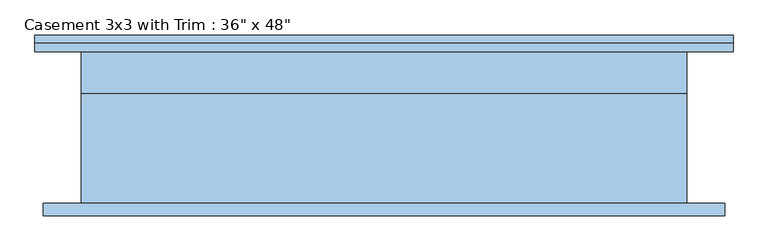
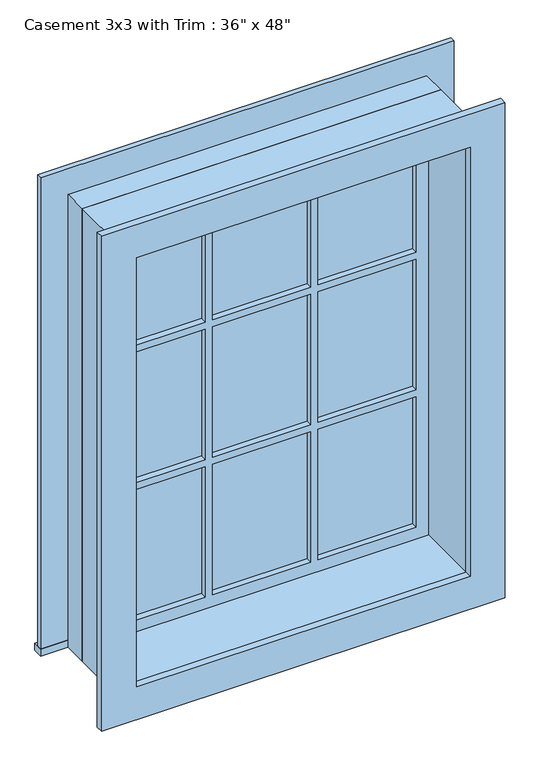
"""IFC4 building model written with IfcOpenShell, lengths in millimetres: window geometry."""

from ifc_helpers import new_model, si_unit, frame, origin, place, context, project, spatial, polyline, outline, extrude, source, transform, mapped, element, save


def window_b7d400b3(model_context):
    return source(origin(), model_context, "Body", "SweptSolid", [
        extrude(outline(polyline([(-527.05, 139.7), (527.05, 139.7), (527.05, 114.3), (-527.05, 114.3), (-527.05, 139.7)])), frame((0.0, 0.0, 914.4), z_axis=(0.0, 0.0, 1.0), x_axis=(1.0, 0.0, 0.0)), (0.0, 0.0, 1.0), 19.05),
        extrude(outline(polyline([(2114.55, -438.15), (2114.55, 438.15), (933.45, 438.15), (933.45, 527.05), (2203.45, 527.05), (2203.45, -527.05), (933.45, -527.05), (933.45, -438.15), (2114.55, -438.15)])), frame((0.0, 114.3, 0.0), z_axis=(0.0, 1.0, 0.0), x_axis=(0.0, 0.0, 1.0)), (0.0, 0.0, 1.0), 12.7),
        extrude(outline(polyline([(143.9333333, 79.375), (393.7, 79.375), (393.7, 66.675), (143.9333333, 66.675), (143.9333333, 79.375)])), frame((0.0, 0.0, 1718.7333333), z_axis=(0.0, 0.0, 1.0), x_axis=(1.0, 0.0, 0.0)), (0.0, 0.0, 1.0), 351.3666667),
        extrude(outline(polyline([(-124.8833333, 79.375), (124.8833333, 79.375), (124.8833333, 66.675), (-124.8833333, 66.675), (-124.8833333, 79.375)])), frame((0.0, 0.0, 1718.7333333), z_axis=(0.0, 0.0, 1.0), x_axis=(1.0, 0.0, 0.0)), (0.0, 0.0, 1.0), 351.3666667),
        extrude(outline(polyline([(-393.7, 79.375), (-143.9333333, 79.375), (-143.9333333, 66.675), (-393.7, 66.675), (-393.7, 79.375)])), frame((0.0, 0.0, 1718.7333333), z_axis=(0.0, 0.0, 1.0), x_axis=(1.0, 0.0, 0.0)), (0.0, 0.0, 1.0), 351.3666667),
        extrude(outline(polyline([(-393.7, 79.375), (-143.9333333, 79.375), (-143.9333333, 66.675), (-393.7, 66.675), (-393.7, 79.375)])), frame((0.0, 0.0, 1348.3166667), z_axis=(0.0, 0.0, 1.0), x_axis=(1.0, 0.0, 0.0)), (0.0, 0.0, 1.0), 351.3666667),
        extrude(outline(polyline([(-124.8833333, 79.375), (124.8833333, 79.375), (124.8833333, 66.675), (-124.8833333, 66.675), (-124.8833333, 79.375)])), frame((0.0, 0.0, 1348.3166667), z_axis=(0.0, 0.0, 1.0), x_axis=(1.0, 0.0, 0.0)), (0.0, 0.0, 1.0), 351.3666667),
        extrude(outline(polyline([(143.9333333, 79.375), (393.7, 79.375), (393.7, 66.675), (143.9333333, 66.675), (143.9333333, 79.375)])), frame((0.0, 0.0, 1348.3166667), z_axis=(0.0, 0.0, 1.0), x_axis=(1.0, 0.0, 0.0)), (0.0, 0.0, 1.0), 351.3666667),
        extrude(outline(polyline([(143.9333333, 79.375), (393.7, 79.375), (393.7, 66.675), (143.9333333, 66.675), (143.9333333, 79.375)])), frame((0.0, 0.0, 977.9), z_axis=(0.0, 0.0, 1.0), x_axis=(1.0, 0.0, 0.0)), (0.0, 0.0, 1.0), 351.3666667),
        extrude(outline(polyline([(-124.8833333, 79.375), (124.8833333, 79.375), (124.8833333, 66.675), (-124.8833333, 66.675), (-124.8833333, 79.375)])), frame((0.0, 0.0, 977.9), z_axis=(0.0, 0.0, 1.0), x_axis=(1.0, 0.0, 0.0)), (0.0, 0.0, 1.0), 351.3666667),
        extrude(outline(polyline([(-393.7, 79.375), (-143.9333333, 79.375), (-143.9333333, 66.675), (-393.7, 66.675), (-393.7, 79.375)])), frame((0.0, 0.0, 977.9), z_axis=(0.0, 0.0, 1.0), x_axis=(1.0, 0.0, 0.0)), (0.0, 0.0, 1.0), 351.3666667),
        extrude(outline(polyline([(2190.75, 514.35), (2190.75, -514.35), (857.25, -514.35), (857.25, 514.35), (2190.75, 514.35)]), holes=[polyline([(2101.85, 425.45), (946.15, 425.45), (946.15, -425.45), (2101.85, -425.45), (2101.85, 425.45)])]), frame((0.0, -133.35, 0.0), z_axis=(0.0, 1.0, 0.0), x_axis=(0.0, 0.0, 1.0)), (0.0, 0.0, 1.0), 19.05),
        extrude(outline(polyline([(2114.55, -438.15), (933.45, -438.15), (933.45, 438.15), (2114.55, 438.15), (2114.55, -438.15)]), holes=[polyline([(2070.1, -143.9333333), (1718.7333333, -143.9333333), (1718.7333333, -393.7), (2070.1, -393.7), (2070.1, -143.9333333)]), polyline([(1699.6833333, -143.9333333), (1348.3166667, -143.9333333), (1348.3166667, -393.7), (1699.6833333, -393.7), (1699.6833333, -143.9333333)]), polyline([(1329.2666667, -143.9333333), (977.9, -143.9333333), (977.9, -393.7), (1329.2666667, -393.7), (1329.2666667, -143.9333333)]), polyline([(2070.1, 124.8833333), (1718.7333333, 124.8833333), (1718.7333333, -124.8833333), (2070.1, -124.8833333), (2070.1, 124.8833333)]), polyline([(1699.6833333, 124.8833333), (1348.3166667, 124.8833333), (1348.3166667, -124.8833333), (1699.6833333, -124.8833333), (1699.6833333, 124.8833333)]), polyline([(1329.2666667, 124.8833333), (977.9, 124.8833333), (977.9, -124.8833333), (1329.2666667, -124.8833333), (1329.2666667, 124.8833333)]), polyline([(2070.1, 393.7), (1718.7333333, 393.7), (1718.7333333, 143.9333333), (2070.1, 143.9333333), (2070.1, 393.7)]), polyline([(1699.6833333, 393.7), (1348.3166667, 393.7), (1348.3166667, 143.9333333), (1699.6833333, 143.9333333), (1699.6833333, 393.7)]), polyline([(1329.2666667, 393.7), (977.9, 393.7), (977.9, 143.9333333), (1329.2666667, 143.9333333), (1329.2666667, 393.7)])]), frame((0.0, 50.8, 0.0), z_axis=(0.0, 1.0, 0.0), x_axis=(0.0, 0.0, 1.0)), (0.0, 0.0, 1.0), 44.45),
        extrude(outline(polyline([(2133.6, -457.2), (914.4, -457.2), (914.4, 457.2), (2133.6, 457.2), (2133.6, -457.2)]), holes=[polyline([(2101.85, -425.45), (2101.85, 425.45), (946.15, 425.45), (946.15, -425.45), (2101.85, -425.45)])]), frame((0.0, -114.3, 0.0), z_axis=(0.0, 1.0, 0.0), x_axis=(0.0, 0.0, 1.0)), (0.0, 0.0, 1.0), 165.1),
        extrude(outline(polyline([(2133.6, 457.2), (2133.6, -457.2), (914.4, -457.2), (914.4, 457.2), (2133.6, 457.2)]), holes=[polyline([(2114.55, 438.15), (933.45, 438.15), (933.45, -438.15), (2114.55, -438.15), (2114.55, 438.15)])]), frame((0.0, 50.8, 0.0), z_axis=(0.0, 1.0, 0.0), x_axis=(0.0, 0.0, 1.0)), (0.0, 0.0, 1.0), 63.5),
    ])


if __name__ == "__main__":
    model = new_model("IFC4")
    model_context = context("Model", 3, world=origin())
    ifc_project = project(units=[si_unit("LENGTHUNIT", "METRE", prefix="MILLI")], contexts=[model_context])
    site = spatial("IfcSite", under=ifc_project)
    building = spatial("IfcBuilding", under=site)
    placement = place(None, origin())
    window_shape = window_b7d400b3(model_context)
    element("IfcWindow", 1, ObjectType="Casement 3x3 with Trim : 36\" x 48\"", at=placement, inside=building, context=model_context, shape_type="MappedRepresentation", body=[
        mapped(window_shape, transform((0.0, 0.0, 0.0), x_axis=(1.0, 0.0, 0.0), y_axis=(0.0, 1.0, 0.0), z_axis=(0.0, 0.0, 1.0))),
    ])
    save(model, "model.ifc")

# Revit data of these elements
# Type "Casement 3x3 with Trim : 36\" x 48\""
#   Type Mark = "10"
#   Construction Type Id = "GSP4R"
#   Assembly Code = "B2020100"
#   Analytic Construction = "1/8 in Pilkington single glazing"
#   Visual Light Transmittance = 0.9
#   Solar Heat Gain Coefficient = 0.78
#   Heat Transfer Coefficient (U) = 0.6496 BTU/(h·ft²·°F)
#   Height = 4' - 0"
#   Default Sill Height = 3' - 0"
#   Trim Projection - Ext. = 0' - 0 1/2"
#   Trim Projection - Int. = 0' - 0 3/4"
#   Trim Width - Exterior = 0' - 3 1/2"
#   Trim Width - Interior = 0' - 3 1/2"
#   Width = 3' - 0"
#   Window Inset = 0' - 0 3/4"
#   Define Thermal Properties by = 1
#   Glass Pane Material = Glass
#   Sash Material = Sash
#   Trim Exterior Material = Trim
#   Trim Interior Material = Trim
#   Wall Closure = (empty or 0)
# Element 1 (IfcWindow, "Casement 3x3 with Trim : 36\" x 48\"")
#   Materials on its faces: "Sash", "Glass", "Trim"
# Materials
#   "Glass": class "Glass", colour RGB 0 128 192, transparency 0.75, Description = "Soda Lime Glass", Cost = 0
#   "Sash": class "Wood", colour RGB 224 178 126, transparency 0
#   "Trim": class "Wood", colour RGB 224 178 126, transparency 0
